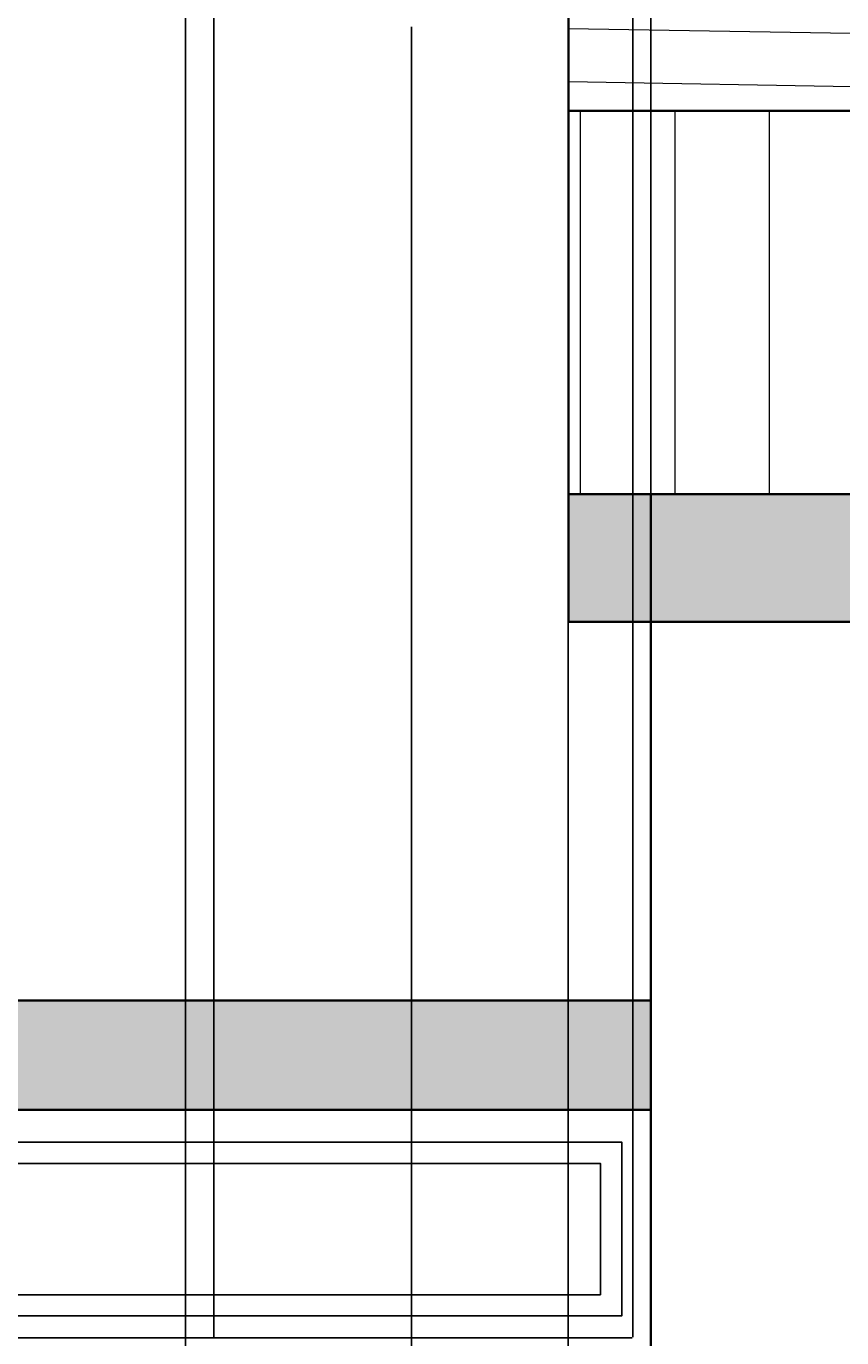
# Model space of a CAD drawing. Units: inches. Extents: x -145 to 510, y 5 to 386.
# Tile 20 of 25: x 259 to 335, y 157 to 280. Entities that reach past the tile are written whole.
import ezdxf

# ---------------------------------------------------------------- set-up
doc = ezdxf.new("R2010")
doc.units = ezdxf.units.IN
doc.header["$MEASUREMENT"] = 0
for name, color, linetype, lineweight in [('A-ANNO-DIMS', 2, 'Continuous', 18), ('A-ELEV', 7, 'Continuous', 35), ('A-ELEV-PATT', 8, 'Continuous', 13), ('A-GLAZ', 4, 'Continuous', 25)]:
    doc.layers.add(name, color=color, linetype=linetype, lineweight=lineweight)
doc.styles.get("Standard").update_dxf_attribs({"font": 'arial.ttf'})
doc.dimstyles.get("Standard").update_dxf_attribs({"dimtxt": 0.6875, "dimasz": 0.18, "dimexe": 0.18, "dimexo": 0.0625, "dimgap": 0.09, "dimtad": 0, "dimtih": 1, "dimtoh": 1, "dimdec": 4, "dimzin": 0, "dimdsep": 46, "dimlunit": 4, "dimtxsty": 'Standard', "dimcen": 0.09, "dimadec": 0, "dimazin": 0, "dimtfac": 1, "dimtdec": 4, "dimtofl": 0, "dimtmove": 0, "dimatfit": 3, "dimfxl": 1, "dimtolj": 1, "dimtzin": 0, "dimarcsym": 0})

# ---------------------------------------------------------------- blocks, each defined once
blk = doc.blocks.new('*D19')
at = {"layer": 'A-ANNO-DIMS', "color": 0, "lineweight": -2, "transparency": 16777216}
for p, q in [((478.76, 355.89), (-144.05, 355.89)), ((-143.87, 355.71), (-143.87, 218.33)), ((-143.87, 80.07), (-143.87, 217.45)), ((-114.04, 79.89), (-144.05, 79.89))]:
    blk.add_line(p, q, dxfattribs=at)
at = {"layer": 'A-ANNO-DIMS', "color": 0, "transparency": 16777216}
for points in [[(-143.9, 355.71), (-143.84, 355.71), (-143.87, 355.89)], [(-143.9, 80.07), (-143.84, 80.07), (-143.87, 79.89)]]:
    blk.add_solid(points, dxfattribs=at)
at = {"layer": 'Defpoints', "color": 0, "transparency": 16777216}
for p in [(-143.87, 355.89), (478.83, 355.89), (-113.97, 79.89)]:
    blk.add_point(p, dxfattribs=at)
at = {"layer": 'A-ANNO-DIMS', "color": 0, "transparency": 16777216, "insert": (-143.87, 217.89), "char_height": 0.688, "attachment_point": 5}
blk.add_mtext('\\A1;276', dxfattribs=at)
blk = doc.blocks.new('*D45')
at = {"layer": 'A-ANNO-DIMS', "color": 0, "lineweight": -2, "transparency": 16777216}
for p, q in [((210.8, 188.37), (210.8, 385.97)), ((210.98, 385.79), (262.53, 385.79)), ((317.05, 385.79), (265.5, 385.79)), ((317.23, 178.08), (317.23, 385.97))]:
    blk.add_line(p, q, dxfattribs=at)
at = {"layer": 'A-ANNO-DIMS', "color": 0, "transparency": 16777216}
for points in [[(210.98, 385.82), (210.98, 385.76), (210.8, 385.79)], [(317.05, 385.82), (317.05, 385.76), (317.23, 385.79)]]:
    blk.add_solid(points, dxfattribs=at)
at = {"layer": 'Defpoints', "color": 0, "transparency": 16777216}
for p in [(317.23, 385.79), (210.8, 188.31), (317.23, 178.02)]:
    blk.add_point(p, dxfattribs=at)
at = {"layer": 'A-ANNO-DIMS', "color": 0, "transparency": 16777216, "insert": (264.01, 385.79), "char_height": 0.688, "attachment_point": 5}
blk.add_mtext('\\A1;106.43', dxfattribs=at)
blk = doc.blocks.new('*D47')
at = {"layer": 'A-ANNO-DIMS', "color": 0, "lineweight": -2, "transparency": 16777216}
for p, q in [((294.74, 279.78), (294.74, 5.19)), ((309.47, 271.83), (309.47, 5.19)), ((294.92, 5.37), (300.62, 5.37)), ((309.29, 5.37), (303.59, 5.37))]:
    blk.add_line(p, q, dxfattribs=at)
at = {"layer": 'A-ANNO-DIMS', "color": 0, "transparency": 16777216}
for points in [[(294.92, 5.4), (294.92, 5.34), (294.74, 5.37)], [(309.29, 5.4), (309.29, 5.34), (309.47, 5.37)]]:
    blk.add_solid(points, dxfattribs=at)
at = {"layer": 'Defpoints', "color": 0, "transparency": 16777216}
for p in [(294.74, 279.84), (309.47, 271.89), (309.47, 5.37)]:
    blk.add_point(p, dxfattribs=at)
at = {"layer": 'A-ANNO-DIMS', "color": 0, "transparency": 16777216, "insert": (302.11, 5.37), "char_height": 0.688, "attachment_point": 5}
blk.add_mtext('\\A1;14.736', dxfattribs=at)
blk = doc.blocks.new('*D48')
at = {"layer": 'A-ANNO-DIMS', "color": 0, "lineweight": -2, "transparency": 16777216}
for p, q in [((309.47, 223.83), (309.47, 5.19)), ((317.23, 223.83), (317.23, 5.19)), ((309.65, 5.37), (312.1, 5.37)), ((317.05, 5.37), (314.6, 5.37))]:
    blk.add_line(p, q, dxfattribs=at)
at = {"layer": 'A-ANNO-DIMS', "color": 0, "transparency": 16777216}
for points in [[(309.65, 5.4), (309.65, 5.34), (309.47, 5.37)], [(317.05, 5.4), (317.05, 5.34), (317.23, 5.37)]]:
    blk.add_solid(points, dxfattribs=at)
at = {"layer": 'Defpoints', "color": 0, "transparency": 16777216}
for p in [(309.47, 223.89), (317.23, 223.89), (317.23, 5.37)]:
    blk.add_point(p, dxfattribs=at)
at = {"layer": 'A-ANNO-DIMS', "color": 0, "transparency": 16777216, "insert": (313.35, 5.37), "char_height": 0.688, "attachment_point": 5}
blk.add_mtext('\\A1;7.753', dxfattribs=at)
blk = doc.blocks.new('*D50')
at = {"layer": 'A-ANNO-DIMS', "color": 0, "lineweight": -2, "transparency": 16777216}
for p, q in [((221.53, 156.67), (221.53, 385.97)), ((221.71, 385.79), (246.26, 385.79)), ((273.31, 385.79), (248.76, 385.79)), ((273.49, 156.67), (273.49, 385.97))]:
    blk.add_line(p, q, dxfattribs=at)
at = {"layer": 'A-ANNO-DIMS', "color": 0, "transparency": 16777216}
for points in [[(221.71, 385.82), (221.71, 385.76), (221.53, 385.79)], [(273.31, 385.82), (273.31, 385.76), (273.49, 385.79)]]:
    blk.add_solid(points, dxfattribs=at)
at = {"layer": 'Defpoints', "color": 0, "transparency": 16777216}
for p in [(273.49, 385.79), (221.53, 156.61), (273.49, 156.61)]:
    blk.add_point(p, dxfattribs=at)
at = {"layer": 'A-ANNO-DIMS', "color": 0, "transparency": 16777216, "insert": (247.51, 385.79), "char_height": 0.688, "attachment_point": 5}
blk.add_mtext('\\A1;51.96', dxfattribs=at)
blk = doc.blocks.new('*D51')
at = {"layer": 'A-ANNO-DIMS', "color": 0, "lineweight": -2, "transparency": 16777216}
for p, q in [((273.31, 385.79), (273.13, 385.79)), ((273.49, 156.67), (273.49, 385.97)), ((276.14, 156.67), (276.14, 385.97)), ((276.32, 385.79), (276.5, 385.79))]:
    blk.add_line(p, q, dxfattribs=at)
at = {"layer": 'A-ANNO-DIMS', "color": 0, "transparency": 16777216}
for points in [[(273.31, 385.82), (273.31, 385.76), (273.49, 385.79)], [(276.32, 385.82), (276.32, 385.76), (276.14, 385.79)]]:
    blk.add_solid(points, dxfattribs=at)
at = {"layer": 'Defpoints', "color": 0, "transparency": 16777216}
for p in [(276.14, 385.79), (273.49, 156.61), (276.14, 156.61)]:
    blk.add_point(p, dxfattribs=at)
at = {"layer": 'A-ANNO-DIMS', "color": 0, "transparency": 16777216, "insert": (274.82, 385.79), "char_height": 0.688, "attachment_point": 5}
blk.add_mtext('\\A1;2.651', dxfattribs=at)
blk = doc.blocks.new('*D52')
at = {"layer": 'A-ANNO-DIMS', "color": 0, "lineweight": -2, "transparency": 16777216}
for p, q in [((276.14, 156.67), (276.14, 385.97)), ((276.32, 385.79), (294.66, 385.79)), ((315.37, 385.79), (297.03, 385.79)), ((315.55, 156.67), (315.55, 385.97))]:
    blk.add_line(p, q, dxfattribs=at)
at = {"layer": 'A-ANNO-DIMS', "color": 0, "transparency": 16777216}
for points in [[(276.32, 385.82), (276.32, 385.76), (276.14, 385.79)], [(315.37, 385.82), (315.37, 385.76), (315.55, 385.79)]]:
    blk.add_solid(points, dxfattribs=at)
at = {"layer": 'Defpoints', "color": 0, "transparency": 16777216}
for p in [(315.55, 385.79), (276.14, 156.61), (315.55, 156.61)]:
    blk.add_point(p, dxfattribs=at)
at = {"layer": 'A-ANNO-DIMS', "color": 0, "transparency": 16777216, "insert": (295.85, 385.79), "char_height": 0.688, "attachment_point": 5}
blk.add_mtext('\\A1;39.41', dxfattribs=at)
blk = doc.blocks.new('*D54')
at = {"layer": 'A-ANNO-DIMS', "color": 0, "lineweight": -2, "transparency": 16777216}
for p, q in [((315.49, 156.61), (-144.05, 156.61)), ((-143.87, 156.43), (-143.87, 121.38)), ((-143.87, 85.44), (-143.87, 120.5)), ((315.49, 85.26), (-144.05, 85.26))]:
    blk.add_line(p, q, dxfattribs=at)
at = {"layer": 'A-ANNO-DIMS', "color": 0, "transparency": 16777216}
for points in [[(-143.9, 156.43), (-143.84, 156.43), (-143.87, 156.61)], [(-143.9, 85.44), (-143.84, 85.44), (-143.87, 85.26)]]:
    blk.add_solid(points, dxfattribs=at)
at = {"layer": 'Defpoints', "color": 0, "transparency": 16777216}
for p in [(-143.87, 156.61), (315.55, 156.61), (315.55, 85.26)]:
    blk.add_point(p, dxfattribs=at)
at = {"layer": 'A-ANNO-DIMS', "color": 0, "transparency": 16777216, "insert": (-143.87, 120.94), "char_height": 0.688, "attachment_point": 5}
blk.add_mtext('\\A1;71.35', dxfattribs=at)
blk = doc.blocks.new('*D55')
at = {"layer": 'A-ANNO-DIMS', "color": 0, "lineweight": -2, "transparency": 16777216}
for p, q in [((314.43, 174.99), (-144.05, 174.99)), ((-143.87, 174.81), (-143.87, 167.27)), ((-143.87, 158.84), (-143.87, 166.38)), ((314.43, 158.66), (-144.05, 158.66))]:
    blk.add_line(p, q, dxfattribs=at)
at = {"layer": 'A-ANNO-DIMS', "color": 0, "transparency": 16777216}
for points in [[(-143.9, 174.81), (-143.84, 174.81), (-143.87, 174.99)], [(-143.9, 158.84), (-143.84, 158.84), (-143.87, 158.66)]]:
    blk.add_solid(points, dxfattribs=at)
at = {"layer": 'Defpoints', "color": 0, "transparency": 16777216}
for p in [(-143.87, 174.99), (314.49, 174.99), (314.49, 158.66)]:
    blk.add_point(p, dxfattribs=at)
at = {"layer": 'A-ANNO-DIMS', "color": 0, "transparency": 16777216, "insert": (-143.87, 166.82), "char_height": 0.688, "attachment_point": 5}
blk.add_mtext('\\A1;16.335', dxfattribs=at)
blk = doc.blocks.new('*D56')
at = {"layer": 'A-ANNO-DIMS', "color": 0, "lineweight": -2, "transparency": 16777216}
for p, q in [((273.49, 156.55), (273.49, 5.19)), ((263.92, 130.61), (263.92, 5.19)), ((264.1, 5.37), (267.46, 5.37)), ((273.31, 5.37), (269.95, 5.37))]:
    blk.add_line(p, q, dxfattribs=at)
at = {"layer": 'A-ANNO-DIMS', "color": 0, "transparency": 16777216}
for points in [[(264.1, 5.4), (264.1, 5.34), (263.92, 5.37)], [(273.31, 5.4), (273.31, 5.34), (273.49, 5.37)]]:
    blk.add_solid(points, dxfattribs=at)
at = {"layer": 'Defpoints', "color": 0, "transparency": 16777216}
for p in [(273.49, 156.61), (263.92, 130.67), (273.49, 5.37)]:
    blk.add_point(p, dxfattribs=at)
at = {"layer": 'A-ANNO-DIMS', "color": 0, "transparency": 16777216, "insert": (268.7, 5.37), "char_height": 0.688, "attachment_point": 5}
blk.add_mtext('\\A1;9.572', dxfattribs=at)

msp = doc.modelspace()

# ---------------------------------------------------------------- hatches: boundary and pattern name
at = {"layer": 'A-ELEV-PATT'}
h = msp.add_hatch(dxfattribs=at)
h.set_pattern_fill('ANSI31', color=256, scale=40, angle=134)
h.paths.add_polyline_path([(478.8263, 355.8905), (309.4739, 355.8905), (309.4739, 341.168), (334.4402, 341.168), (334.4402, 327.6093), (309.4739, 327.6093), (309.4739, 271.8905), (478.8263, 271.8905)])
h.paths.add_polyline_path([(442.9009, 301.8821), (351.234, 301.8821), (351.234, 332.4358), (442.9009, 332.4358)], flags=16)
h.paths.add_polyline_path([(440.9009, 303.8821), (353.234, 303.8821), (353.234, 330.4358), (440.9009, 330.4358)], flags=0)
h = msp.add_hatch(color=256, dxfattribs=at)
h.dxf.hatch_style = 1
h.paths.add_polyline_path([(334.4402, 341.168), (69.7763, 341.168), (69.7763, 327.6093), (334.4402, 327.6093)])
h.paths.add_polyline_path([(69.7763, 341.168), (34.2706, 341.168), (34.2706, 327.6093), (69.7763, 327.6093)])
h.paths.add_polyline_path([(317.2273, 188.3087), (210.7973, 188.3087), (210.7973, 178.0195), (317.2273, 178.0195)])
h.paths.add_polyline_path([(474.4893, 235.8905), (317.2273, 235.8905), (317.2273, 223.8905), (474.4893, 223.8905)])
h.paths.add_polyline_path([(317.2273, 235.8905), (309.4739, 235.8905), (309.4739, 223.8905), (317.2273, 223.8905)])
h.paths.add_polyline_path([(478.8263, 235.8905), (474.4893, 235.8905), (474.4893, 223.8905), (478.8263, 223.8905)])
h = msp.add_hatch(dxfattribs=at)
h.set_pattern_fill('ANSI31', color=256, scale=71, angle=45)
h.paths.add_polyline_path([(478.8263, 271.8905), (309.4739, 271.8905), (309.4739, 259.8905), (309.4739, 235.8905), (317.2273, 235.8905), (474.4893, 235.8905), (478.8263, 235.8905)])

# ---------------------------------------------------------------- linework, layer by layer
at = {"layer": 'A-ELEV'}
for p, q in [((309.4739, 271.8905), (309.4739, 327.6093)), ((309.4739, 259.8905), (309.4739, 271.8905)), ((309.4739, 271.8905), (478.8263, 271.8905)), ((309.4739, 235.8905), (309.4739, 259.8905)), ((317.2273, 235.8905), (309.4739, 235.8905)), ((309.4739, 235.8905), (309.4739, 223.8905)), ((317.2273, 223.8905), (317.2273, 235.8905)), ((317.2273, 235.8905), (474.4893, 235.8905)), ((309.4739, 223.8905), (317.2273, 223.8905)), ((317.2273, 79.8905), (317.2273, 223.8905)), ((317.2273, 223.8905), (474.4893, 223.8905)), ((210.7973, 188.3087), (317.2273, 188.3087)), ((210.7973, 178.0195), (317.2273, 178.0195))]:
    msp.add_line(p, q, dxfattribs=at)
at = {"layer": 'A-GLAZ'}
for points in [[(221.5292, 174.9923), (314.494, 174.9923), (314.494, 158.657), (221.5292, 158.657)], [(223.5292, 172.9923), (312.494, 172.9923), (312.494, 160.657), (223.5292, 160.657)]]:
    msp.add_lwpolyline(points, close=True, dxfattribs=at)

# ---------------------------------------------------------------- dimensions: what is measured, and where the dimension line sits
at = {"layer": 'A-ANNO-DIMS'}
for base, p1, p2, override, picture, middle in [((317.2273, 385.7905), (210.7973, 188.3087), (317.2273, 178.0195), {"dimdec": 2, "dimlfac": 1, "dimrnd": 0, "dimzin": 0, "dimdsep": 46, "dimlunit": 2}, '*D45', (264.0123, 385.7905)), ((273.4905, 385.7905), (221.5292, 156.6093), (273.4905, 156.6093), {"dimdec": 2, "dimlfac": 1, "dimrnd": 0, "dimzin": 0, "dimdsep": 46, "dimlunit": 2}, '*D50', (247.5098, 385.7905)), ((276.1416, 385.7905), (273.4905, 156.6093), (276.1416, 156.6093), {"dimdec": 3, "dimlfac": 1, "dimrnd": 0, "dimzin": 0, "dimdsep": 46, "dimlunit": 2}, '*D51', (274.8161, 385.7905)), ((315.5545, 385.7905), (276.1416, 156.6093), (315.5545, 156.6093), {"dimdec": 2, "dimlfac": 1, "dimrnd": 0, "dimzin": 0, "dimdsep": 46, "dimlunit": 2}, '*D52', (295.848, 385.7905)), ((309.4739, 5.3738), (294.738, 279.8443), (309.4739, 271.8905), {"dimdec": 3, "dimlfac": 1, "dimrnd": 0, "dimzin": 0, "dimdsep": 46, "dimlunit": 2}, '*D47', (302.106, 5.3738)), ((317.2273, 5.3738), (309.4739, 223.8905), (317.2273, 223.8905), {"dimdec": 3, "dimlfac": 1, "dimrnd": 0, "dimzin": 0, "dimdsep": 46, "dimlunit": 2}, '*D48', (313.3506, 5.3738)), ((273.4905, 5.3738), (263.9183, 130.6707), (273.4905, 156.6093), {"dimdec": 3, "dimlfac": 1, "dimrnd": 0, "dimzin": 0, "dimdsep": 46, "dimlunit": 2}, '*D56', (268.7044, 5.3738))]:
    dim = msp.add_linear_dim(base=base, p1=p1, p2=p2, dimstyle='Standard', override=override, dxfattribs=at)
    dim.commit()
    dim.dimension.update_dxf_attribs({"geometry": picture, "text_midpoint": middle})
for base, p1, p2, override, picture, middle in [((-143.8737, 355.8905), (-113.9737, 79.8905), (478.8263, 355.8905), {"dimdec": 0, "dimlfac": 1, "dimrnd": 0, "dimzin": 0, "dimdsep": 46, "dimlunit": 2}, '*D19', (-143.8737, 217.8905)), ((-143.8737, 174.9923), (314.494, 158.657), (314.494, 174.9923), {"dimdec": 3, "dimlfac": 1, "dimrnd": 0, "dimzin": 0, "dimdsep": 46, "dimlunit": 2}, '*D55', (-143.8737, 166.8247)), ((-143.8737, 156.6093), (315.5545, 85.2638), (315.5545, 156.6093), {"dimdec": 2, "dimlfac": 1, "dimrnd": 0, "dimzin": 0, "dimdsep": 46, "dimlunit": 2}, '*D54', (-143.8737, 120.9365))]:
    dim = msp.add_linear_dim(base=base, p1=p1, p2=p2, angle=90, dimstyle='Standard', override=override, dxfattribs=at)
    dim.commit()
    dim.dimension.update_dxf_attribs({"geometry": picture, "text_midpoint": middle})

doc.saveas('drawing.dxf')
